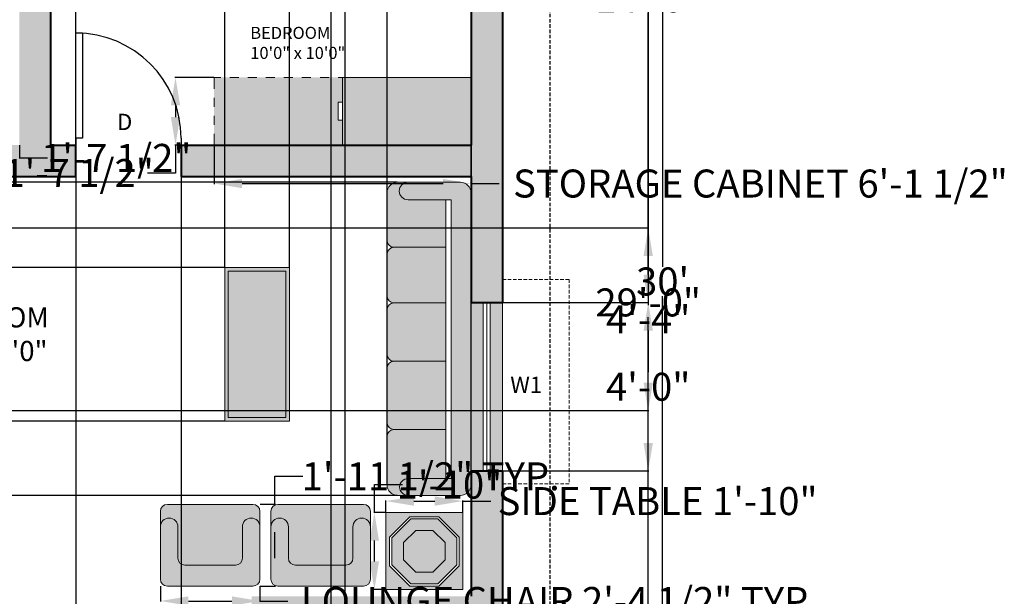
# Model space of a CAD drawing. Units: inches. Extents: x 277 to 728, y 649 to 1132.
# Tile 3 of 4: x 447 to 728, y 813 to 978. Entities that reach past the tile are written whole.
import ezdxf

# ---------------------------------------------------------------- set-up
doc = ezdxf.new("R2010")
doc.units = ezdxf.units.IN
doc.header["$MEASUREMENT"] = 0
doc.linetypes.add('DASHEDX2', pattern=[1.5, 1, -0.5])
for name, color, linetype, lineweight in [('A-ANNO-DIMS', 2, 'Continuous', 18), ('A-ANNO-TEXT', 7, 'Continuous', 18), ('A-AREA-IDEN', 7, 'Continuous', 25), ('A-DOOR', 3, 'Continuous', 25), ('A-FURN', 8, 'Continuous', 18), ('A-GLAZ', 4, 'Continuous', 18), ('A-GLAZ-OVHD', 8, 'DASHEDX2', 13), ('A-WALL', 7, 'Continuous', 40), ('A-WALL-PATT', 8, 'Continuous', 13), ('C-PROP', 7, 'DASHEDX2', 25)]:
    doc.layers.add(name, color=color, linetype=linetype, lineweight=lineweight)
doc.layers.add('A-FURN-PATT', color=9, linetype='Continuous', lineweight=9, true_color=0xd6bdce)
doc.layers.add('A-GLAZ-PATT', color=144, linetype='Continuous', lineweight=13, true_color=0x1e788f)
doc.styles.get("Standard").update_dxf_attribs({"font": 'arial.ttf'})
doc.dimstyles.get("Standard").update_dxf_attribs({"dimtxt": 8, "dimasz": 8, "dimexe": 0.18, "dimexo": 0.0625, "dimgap": 0.09, "dimtad": 0, "dimtih": 1, "dimtoh": 1, "dimdec": 0, "dimzin": 0, "dimdsep": 46, "dimlunit": 3, "dimtxsty": 'Standard', "dimcen": 0.09, "dimadec": 0, "dimazin": 0, "dimtfac": 1, "dimtdec": 0, "dimtofl": 0, "dimtmove": 0, "dimatfit": 3, "dimfxl": 1, "dimtolj": 1, "dimtzin": 0, "dimarcsym": 0})

# ---------------------------------------------------------------- blocks, each defined once
blk = doc.blocks.new('*U5')
for p, q in [((0, 0), (0, -6)), ((28, 0), (28, -6))]:
    blk.add_line(p, q)
blk.add_lwpolyline([(0, 0), (0, 28), (1.75, 28), (1.75, 0)], close=True)
blk.add_arc((0, 0), 28, 0, 90)
blk = doc.blocks.new('File Cabinet - Letter')
for p, q in [((0, 0), (15, 0)), ((0, -28.5), (0, 0)), ((15, 0), (15, -28.5)), ((15, -28.5), (0, -28.5)), ((0, -29.5), (0, -28.5)), ((5.5, -28.5), (5.5, -29.5)), ((5.5, -29.5), (9.5, -29.5)), ((9.5, -29.5), (9.5, -28.5)), ((15, -30.5), (15, -32.5)), ((0, -33.5), (0, -31.5)), ((15, -34.5), (15, -36.5)), ((0, -37.5), (0, -35.5)), ((15, -38.5), (15, -40.5)), ((0, -41.5), (0, -39.5)), ((0, -45.5), (0, -43.5)), ((15, -42.5), (15, -44.5)), ((0, -49.5), (0, -47.5)), ((15, -46.5), (15, -48.5)), ((0, -53.5), (0, -51.5)), ((15, -50.5), (15, -52.5)), ((15, -54.5), (15, -57)), ((0, -57), (0, -55.5)), ((2.5, -57), (0, -57)), ((6.5, -57), (4.5, -57)), ((10.5, -57), (8.5, -57)), ((15, -57), (12.5, -57))]:
    blk.add_line(p, q)
blk = doc.blocks.new('Hot Tub')
for p, q in [((0, 0), (0, 69.12)), ((0, 69.12), (69.12, 69.12)), ((21.601, 65.456), (3.272, 47.128)), ((22.464, 63.396), (5.358, 46.29)), ((47.521, 65.456), (21.601, 65.456)), ((46.656, 63.396), (22.464, 63.396)), ((63.763, 46.29), (46.656, 63.396)), ((65.849, 47.128), (47.521, 65.456)), ((69.12, 69.12), (69.12, 0)), ((3.272, 47.128), (3.272, 21.208)), ((5.358, 46.29), (5.358, 22.098)), ((26.785, 53.097), (15.788, 42.101)), ((42.337, 53.097), (26.785, 53.097)), ((53.333, 42.101), (42.337, 53.097)), ((63.763, 22.098), (63.763, 46.29)), ((65.849, 21.208), (65.849, 47.128)), ((15.788, 42.101), (15.788, 26.549)), ((53.333, 26.549), (53.333, 42.101)), ((3.272, 21.208), (21.601, 2.88)), ((5.358, 22.098), (22.464, 4.992)), ((15.788, 26.549), (26.785, 15.552)), ((42.337, 15.552), (53.333, 26.549)), ((46.656, 4.992), (63.763, 22.098)), ((47.521, 2.88), (65.849, 21.208)), ((26.785, 15.552), (42.337, 15.552)), ((69.12, 0), (0, 0)), ((21.601, 2.88), (47.521, 2.88)), ((22.464, 4.992), (46.656, 4.992))]:
    blk.add_line(p, q)
blk = doc.blocks.new('*D21')
at = {"layer": 'A-ANNO-DIMS', "color": 0, "lineweight": -2, "transparency": 16777216}
for p, q in [((598.28, 1083.05), (630.62, 1083.05)), ((630.44, 1075.05), (630.44, 907.23)), ((630.44, 731.05), (630.44, 898.87)), ((598.28, 723.05), (630.62, 723.05))]:
    blk.add_line(p, q, dxfattribs=at)
at = {"layer": 'A-ANNO-DIMS', "color": 0, "transparency": 16777216}
for points in [[(629.11, 1075.05), (631.77, 1075.05), (630.44, 1083.05)], [(629.11, 731.05), (631.77, 731.05), (630.44, 723.05)]]:
    blk.add_solid(points, dxfattribs=at)
at = {"layer": 'Defpoints', "color": 0, "transparency": 16777216}
for p in [(598.22, 1083.05), (598.22, 723.05), (630.44, 723.05)]:
    blk.add_point(p, dxfattribs=at)
at = {"layer": 'A-ANNO-DIMS', "color": 0, "transparency": 16777216, "insert": (630.44, 903.05), "char_height": 8, "attachment_point": 5}
blk.add_mtext("\\A1;30'", dxfattribs=at)
blk = doc.blocks.new('CHAIR-LOUNGE')
h = blk.add_hatch(color=256)
h.dxf.hatch_style = 1
h.paths.add_polyline_path([(23.44, 16.96, -1), (28.44, 16.96), (28.44, 21.37, 0.414214), (26.44, 23.37), (2, 23.37, 0.414214), (0, 21.37), (0, 16.96, -1), (5, 16.96), (5, 8, 0.414214), (7, 6), (21.44, 6, 0.414214), (23.44, 8)])
h = blk.add_hatch(color=256)
h.dxf.hatch_style = 1
h.paths.add_polyline_path([(0, 2, 0.414214), (2, 0), (26.44, 0, 0.414214), (28.44, 2), (28.44, 16.96, 1), (23.44, 16.96), (23.44, 8, -0.414214), (21.44, 6), (7, 6, -0.414214), (5, 8), (5, 16.96, 1), (0, 16.96)])
for p, q in [((2, 23.37), (26.44, 23.37)), ((0, 16.96), (0, 21.37)), ((28.44, 21.37), (28.44, 16.96)), ((0, 16.96), (0, 2)), ((5, 8), (5, 16.96)), ((23.44, 16.96), (23.44, 8)), ((28.44, 2), (28.44, 16.96)), ((21.44, 6), (7, 6)), ((2, 0), (26.44, 0))]:
    blk.add_line(p, q)
for centre, radius, start, end in [((2, 21.37), 2, 90, 180), ((26.44, 21.37), 2, 0, 90), ((2.5, 16.96), 2.5, 0, 180), ((25.94, 16.96), 2.5, 0, 180), ((7, 8), 2, 180, 270), ((21.44, 8), 2, 270, 0), ((2, 2), 2, 180, 270), ((26.44, 2), 2, 270, 0)]:
    blk.add_arc(centre, radius, start, end)
blk = doc.blocks.new('*D25')
at = {"layer": 'A-ANNO-DIMS', "color": 0, "lineweight": -2, "transparency": 16777216}
for p, q in [((551.4, 837.04), (551.4, 840.45)), ((559.4, 840.27), (565.36, 840.27)), ((573.36, 837.04), (573.36, 840.45)), ((573.36, 840.27), (581.36, 840.27))]:
    blk.add_line(p, q, dxfattribs=at)
at = {"layer": 'A-ANNO-DIMS', "color": 0, "transparency": 16777216}
for points in [[(559.4, 841.6), (559.4, 838.94), (551.4, 840.27)], [(565.36, 841.6), (565.36, 838.94), (573.36, 840.27)]]:
    blk.add_solid(points, dxfattribs=at)
at = {"layer": 'Defpoints', "color": 0, "transparency": 16777216}
for p in [(573.36, 840.27), (551.4, 836.98), (573.36, 836.98)]:
    blk.add_point(p, dxfattribs=at)
at = {"layer": 'A-ANNO-DIMS', "color": 0, "transparency": 16777216, "insert": (629.02, 840.27), "char_height": 8, "attachment_point": 5}
blk.add_mtext('\\A1;SIDE TABLE 1\'-10"', dxfattribs=at)
blk = doc.blocks.new('*D26')
at = {"layer": 'A-ANNO-DIMS', "color": 0, "lineweight": -2, "transparency": 16777216}
for p, q in [((548.11, 836.98), (548.11, 844.98)), ((548.11, 844.98), (556.11, 844.98)), ((551.34, 836.98), (547.93, 836.98)), ((548.11, 823.02), (548.11, 828.98)), ((551.34, 815.02), (547.93, 815.02))]:
    blk.add_line(p, q, dxfattribs=at)
at = {"layer": 'A-ANNO-DIMS', "color": 0, "transparency": 16777216}
for points in [[(546.77, 828.98), (549.44, 828.98), (548.11, 836.98)], [(546.77, 823.02), (549.44, 823.02), (548.11, 815.02)]]:
    blk.add_solid(points, dxfattribs=at)
at = {"layer": 'Defpoints', "color": 0, "transparency": 16777216}
for p in [(548.11, 836.98), (551.4, 836.98), (551.4, 815.02)]:
    blk.add_point(p, dxfattribs=at)
at = {"layer": 'A-ANNO-DIMS', "color": 0, "transparency": 16777216, "insert": (569.56, 844.98), "char_height": 8, "attachment_point": 5}
blk.add_mtext('\\A1;1\'-10"', dxfattribs=at)
blk = doc.blocks.new('*D29')
at = {"layer": 'A-ANNO-DIMS', "color": 0, "lineweight": -2, "transparency": 16777216}
for p, q in [((486.97, 815.91), (486.97, 811.53)), ((515.41, 815.91), (515.41, 811.53)), ((494.97, 811.71), (507.41, 811.71)), ((515.41, 811.71), (523.41, 811.71))]:
    blk.add_line(p, q, dxfattribs=at)
at = {"layer": 'A-ANNO-DIMS', "color": 0, "transparency": 16777216}
for points in [[(494.97, 813.04), (494.97, 810.37), (486.97, 811.71)], [(507.41, 813.04), (507.41, 810.37), (515.41, 811.71)]]:
    blk.add_solid(points, dxfattribs=at)
at = {"layer": 'Defpoints', "color": 0, "transparency": 16777216}
for p in [(486.97, 815.97), (515.41, 815.97), (515.41, 811.71)]:
    blk.add_point(p, dxfattribs=at)
at = {"layer": 'A-ANNO-DIMS', "color": 0, "transparency": 16777216, "insert": (601.11, 811.71), "char_height": 8, "attachment_point": 5}
blk.add_mtext('\\A1;LOUNGE CHAIR 2\'-4 1/2" TYP.', dxfattribs=at)
blk = doc.blocks.new('*D30')
at = {"layer": 'A-ANNO-DIMS', "color": 0, "lineweight": -2, "transparency": 16777216}
for p, q in [((519.67, 839.35), (519.67, 847.35)), ((519.67, 847.35), (527.67, 847.35)), ((515.47, 839.35), (519.85, 839.35)), ((519.67, 823.97), (519.67, 831.35)), ((515.47, 815.97), (519.85, 815.97))]:
    blk.add_line(p, q, dxfattribs=at)
at = {"layer": 'A-ANNO-DIMS', "color": 0, "transparency": 16777216}
for points in [[(518.34, 831.35), (521.01, 831.35), (519.67, 839.35)], [(518.34, 823.97), (521.01, 823.97), (519.67, 815.97)]]:
    blk.add_solid(points, dxfattribs=at)
at = {"layer": 'Defpoints', "color": 0, "transparency": 16777216}
for p in [(515.41, 839.35), (519.67, 839.35), (515.41, 815.97)]:
    blk.add_point(p, dxfattribs=at)
at = {"layer": 'A-ANNO-DIMS', "color": 0, "transparency": 16777216, "insert": (564.2, 847.35), "char_height": 8, "attachment_point": 5}
blk.add_mtext('\\A1;1\'-11 1/2" TYP.', dxfattribs=at)
blk = doc.blocks.new('*D32')
at = {"layer": 'A-ANNO-DIMS', "color": 0, "lineweight": -2, "transparency": 16777216}
for p, q in [((427.01, 942.02), (427, 938.24)), ((446.72, 941.99), (446.71, 938.2)), ((435, 938.4), (438.71, 938.4)), ((446.71, 938.38), (454.71, 938.37))]:
    blk.add_line(p, q, dxfattribs=at)
at = {"layer": 'A-ANNO-DIMS', "color": 0, "transparency": 16777216}
for points in [[(435, 939.74), (435, 937.07), (427, 938.42)], [(438.71, 939.73), (438.71, 937.06), (446.71, 938.38)]]:
    blk.add_solid(points, dxfattribs=at)
at = {"layer": 'Defpoints', "color": 0, "transparency": 16777216}
for p in [(427.01, 942.09), (446.72, 942.05), (446.71, 938.38)]:
    blk.add_point(p, dxfattribs=at)
at = {"layer": 'A-ANNO-DIMS', "color": 0, "transparency": 16777216, "insert": (474.38, 938.37), "char_height": 8, "attachment_point": 5}
blk.add_mtext('\\A1;1\'-7 1/2"', dxfattribs=at)
blk = doc.blocks.new('*D39')
at = {"layer": 'A-ANNO-DIMS', "color": 0, "lineweight": -2, "transparency": 16777216}
for p, q in [((502.31, 941.99), (502.31, 930.86)), ((575.72, 941.99), (575.72, 930.86)), ((510.31, 931.04), (567.72, 931.04)), ((575.72, 931.04), (583.72, 931.04))]:
    blk.add_line(p, q, dxfattribs=at)
at = {"layer": 'A-ANNO-DIMS', "color": 0, "transparency": 16777216}
for points in [[(510.31, 932.37), (510.31, 929.71), (502.31, 931.04)], [(567.72, 932.37), (567.72, 929.71), (575.72, 931.04)]]:
    blk.add_solid(points, dxfattribs=at)
at = {"layer": 'Defpoints', "color": 0, "transparency": 16777216}
for p in [(502.31, 942.05), (575.72, 942.05), (575.72, 931.04)]:
    blk.add_point(p, dxfattribs=at)
at = {"layer": 'A-ANNO-DIMS', "color": 0, "transparency": 16777216, "insert": (658.39, 931.04), "char_height": 8, "attachment_point": 5}
blk.add_mtext('\\A1;STORAGE CABINET 6\'-1 1/2"', dxfattribs=at)
blk = doc.blocks.new('*D40')
at = {"layer": 'A-ANNO-DIMS', "color": 0, "lineweight": -2, "transparency": 16777216}
for p, q in [((502.25, 961.37), (491.12, 961.37)), ((491.3, 953.37), (491.3, 950.05)), ((502.25, 942.05), (491.12, 942.05)), ((491.3, 942.05), (491.3, 934.05)), ((491.3, 934.05), (483.3, 934.05))]:
    blk.add_line(p, q, dxfattribs=at)
at = {"layer": 'A-ANNO-DIMS', "color": 0, "transparency": 16777216}
for points in [[(489.96, 953.37), (492.63, 953.37), (491.3, 961.37)], [(489.96, 950.05), (492.63, 950.05), (491.3, 942.05)]]:
    blk.add_solid(points, dxfattribs=at)
at = {"layer": 'Defpoints', "color": 0, "transparency": 16777216}
for p in [(502.31, 961.37), (491.3, 942.05), (502.31, 942.05)]:
    blk.add_point(p, dxfattribs=at)
at = {"layer": 'A-ANNO-DIMS', "color": 0, "transparency": 16777216, "insert": (463.63, 934.05), "char_height": 8, "attachment_point": 5}
blk.add_mtext('\\A1;1\'-7 1/2"', dxfattribs=at)
blk = doc.blocks.new('*D41')
at = {"layer": 'A-ANNO-DIMS', "color": 0, "lineweight": -2, "transparency": 16777216}
for p, q in [((505.29, 907.01), (299.63, 907.01)), ((299.81, 899.01), (299.81, 889.26)), ((299.81, 871.15), (299.81, 880.9)), ((505.29, 863.15), (299.63, 863.15))]:
    blk.add_line(p, q, dxfattribs=at)
at = {"layer": 'A-ANNO-DIMS', "color": 0, "transparency": 16777216}
for points in [[(298.48, 899.01), (301.15, 899.01), (299.81, 907.01)], [(298.48, 871.15), (301.15, 871.15), (299.81, 863.15)]]:
    blk.add_solid(points, dxfattribs=at)
at = {"layer": 'Defpoints', "color": 0, "transparency": 16777216}
for p in [(299.81, 907.01), (505.35, 907.01), (505.35, 863.15)]:
    blk.add_point(p, dxfattribs=at)
at = {"layer": 'A-ANNO-DIMS', "color": 0, "transparency": 16777216, "insert": (299.81, 885.08), "char_height": 8, "attachment_point": 5}
blk.add_mtext('\\A1;3\'-8"', dxfattribs=at)
blk = doc.blocks.new('*D42')
at = {"layer": 'A-ANNO-DIMS', "color": 0, "lineweight": -2, "transparency": 16777216}
for p, q in [((505.35, 907.07), (505.35, 1117.22)), ((513.35, 1117.04), (515.86, 1117.04)), ((523.86, 907.07), (523.86, 1117.22)), ((523.86, 1117.04), (531.86, 1117.04))]:
    blk.add_line(p, q, dxfattribs=at)
at = {"layer": 'A-ANNO-DIMS', "color": 0, "transparency": 16777216}
for points in [[(513.35, 1118.37), (513.35, 1115.71), (505.35, 1117.04)], [(515.86, 1118.37), (515.86, 1115.71), (523.86, 1117.04)]]:
    blk.add_solid(points, dxfattribs=at)
at = {"layer": 'Defpoints', "color": 0, "transparency": 16777216}
for p in [(523.86, 1117.04), (505.35, 907.01), (523.86, 907.01)]:
    blk.add_point(p, dxfattribs=at)
at = {"layer": 'A-ANNO-DIMS', "color": 0, "transparency": 16777216, "insert": (551.53, 1117.04), "char_height": 8, "attachment_point": 5}
blk.add_mtext('\\A1;1\'-6 1/2"', dxfattribs=at)
blk = doc.blocks.new('*D43')
at = {"layer": 'A-ANNO-DIMS', "color": 0, "lineweight": -2, "transparency": 16777216}
for p, q in [((554.66, 931.4), (299.63, 931.4)), ((299.81, 923.4), (299.81, 890.87)), ((299.81, 849.9), (299.81, 882.42)), ((554.66, 841.9), (299.63, 841.9))]:
    blk.add_line(p, q, dxfattribs=at)
at = {"layer": 'A-ANNO-DIMS', "color": 0, "transparency": 16777216}
for points in [[(298.48, 923.4), (301.15, 923.4), (299.81, 931.4)], [(298.48, 849.9), (301.15, 849.9), (299.81, 841.9)]]:
    blk.add_solid(points, dxfattribs=at)
at = {"layer": 'Defpoints', "color": 0, "transparency": 16777216}
for p in [(299.81, 931.4), (554.72, 931.4), (554.72, 841.9)]:
    blk.add_point(p, dxfattribs=at)
at = {"layer": 'A-ANNO-DIMS', "color": 0, "transparency": 16777216, "insert": (299.81, 886.65), "char_height": 8, "attachment_point": 5}
blk.add_mtext('\\A1;7\'-5 1/2"', dxfattribs=at)
blk = doc.blocks.new('*D44')
at = {"layer": 'A-ANNO-DIMS', "color": 0, "lineweight": -2, "transparency": 16777216}
for p, q in [((543.72, 1117.04), (535.72, 1117.04)), ((551.72, 844.96), (551.72, 1117.22)), ((575.72, 844.96), (575.72, 1117.22)), ((583.72, 1117.04), (591.72, 1117.04))]:
    blk.add_line(p, q, dxfattribs=at)
at = {"layer": 'A-ANNO-DIMS', "color": 0, "transparency": 16777216}
for points in [[(543.72, 1118.37), (543.72, 1115.71), (551.72, 1117.04)], [(583.72, 1118.37), (583.72, 1115.71), (575.72, 1117.04)]]:
    blk.add_solid(points, dxfattribs=at)
at = {"layer": 'Defpoints', "color": 0, "transparency": 16777216}
for p in [(575.72, 1117.04), (551.72, 844.9), (575.72, 844.9)]:
    blk.add_point(p, dxfattribs=at)
at = {"layer": 'A-ANNO-DIMS', "color": 0, "transparency": 16777216, "insert": (563.72, 1117.04), "char_height": 8, "attachment_point": 5}
blk.add_mtext('\\A1;2\'-0"', dxfattribs=at)
blk = doc.blocks.new('*D45')
at = {"layer": 'A-ANNO-DIMS', "color": 0, "lineweight": -2, "transparency": 16777216}
for p, q in [((363.23, 918.34), (626.51, 918.34)), ((626.33, 910.34), (626.33, 896.32)), ((626.33, 874.12), (626.33, 888.14)), ((363.23, 866.12), (626.51, 866.12))]:
    blk.add_line(p, q, dxfattribs=at)
at = {"layer": 'A-ANNO-DIMS', "color": 0, "transparency": 16777216}
for points in [[(625, 910.34), (627.67, 910.34), (626.33, 918.34)], [(625, 874.12), (627.67, 874.12), (626.33, 866.12)]]:
    blk.add_solid(points, dxfattribs=at)
at = {"layer": 'Defpoints', "color": 0, "transparency": 16777216}
for p in [(363.17, 918.34), (626.33, 918.34), (363.17, 866.12)]:
    blk.add_point(p, dxfattribs=at)
at = {"layer": 'A-ANNO-DIMS', "color": 0, "transparency": 16777216, "insert": (626.33, 892.23), "char_height": 8, "attachment_point": 5}
blk.add_mtext('\\A1;4\'-4"', dxfattribs=at)
blk = doc.blocks.new('*D48')
at = {"layer": 'A-ANNO-DIMS', "color": 0, "lineweight": -2, "transparency": 16777216}
for p, q in [((584.78, 1071.05), (626.51, 1071.05)), ((626.33, 1063.05), (626.33, 901.23)), ((626.33, 731.05), (626.33, 892.88)), ((584.78, 723.05), (626.51, 723.05))]:
    blk.add_line(p, q, dxfattribs=at)
at = {"layer": 'A-ANNO-DIMS', "color": 0, "transparency": 16777216}
for points in [[(625, 1063.05), (627.67, 1063.05), (626.33, 1071.05)], [(625, 731.05), (627.67, 731.05), (626.33, 723.05)]]:
    blk.add_solid(points, dxfattribs=at)
at = {"layer": 'Defpoints', "color": 0, "transparency": 16777216}
for p in [(584.72, 1071.05), (626.33, 1071.05), (584.72, 723.05)]:
    blk.add_point(p, dxfattribs=at)
at = {"layer": 'A-ANNO-DIMS', "color": 0, "transparency": 16777216, "insert": (626.33, 897.05), "char_height": 8, "attachment_point": 5}
blk.add_mtext('\\A1;29\'-0"', dxfattribs=at)
blk = doc.blocks.new('*D53')
at = {"layer": 'A-ANNO-DIMS', "color": 0, "lineweight": -2, "transparency": 16777216}
for p, q in [((584.78, 897), (626.51, 897)), ((626.33, 889), (626.33, 877.13)), ((626.33, 856.91), (626.33, 868.78)), ((584.78, 848.91), (626.51, 848.91))]:
    blk.add_line(p, q, dxfattribs=at)
at = {"layer": 'A-ANNO-DIMS', "color": 0, "transparency": 16777216}
for points in [[(625, 889), (627.67, 889), (626.33, 897)], [(625, 856.91), (627.67, 856.91), (626.33, 848.91)]]:
    blk.add_solid(points, dxfattribs=at)
at = {"layer": 'Defpoints', "color": 0, "transparency": 16777216}
for p in [(584.72, 897), (626.33, 897), (584.72, 848.91)]:
    blk.add_point(p, dxfattribs=at)
at = {"layer": 'A-ANNO-DIMS', "color": 0, "transparency": 16777216, "insert": (626.33, 872.95), "char_height": 8, "attachment_point": 5}
blk.add_mtext('\\A1;4\'-0"', dxfattribs=at)
blk = doc.blocks.new('*D54')
at = {"layer": 'A-ANNO-DIMS', "color": 0, "lineweight": -2, "transparency": 16777216}
for p, q in [((584.78, 1071.05), (626.51, 1071.05)), ((626.33, 1063.05), (626.33, 988.2)), ((626.33, 905), (626.33, 979.85)), ((584.78, 897), (626.51, 897))]:
    blk.add_line(p, q, dxfattribs=at)
at = {"layer": 'A-ANNO-DIMS', "color": 0, "transparency": 16777216}
for points in [[(625, 1063.05), (627.67, 1063.05), (626.33, 1071.05)], [(625, 905), (627.67, 905), (626.33, 897)]]:
    blk.add_solid(points, dxfattribs=at)
at = {"layer": 'Defpoints', "color": 0, "transparency": 16777216}
for p in [(584.72, 1071.05), (626.33, 1071.05), (584.72, 897)]:
    blk.add_point(p, dxfattribs=at)
at = {"layer": 'A-ANNO-DIMS', "color": 0, "transparency": 16777216, "insert": (626.33, 984.02), "char_height": 8, "attachment_point": 5}
blk.add_mtext('\\A1;14\'-6"', dxfattribs=at)
blk = doc.blocks.new('*D62')
at = {"layer": 'A-ANNO-DIMS', "color": 0, "lineweight": -2, "transparency": 16777216}
for p, q in [((462.81, 941.99), (462.81, 661.09)), ((492.89, 941.99), (492.89, 661.09)), ((454.81, 661.27), (446.81, 661.27)), ((500.89, 661.27), (508.89, 661.27))]:
    blk.add_line(p, q, dxfattribs=at)
at = {"layer": 'A-ANNO-DIMS', "color": 0, "transparency": 16777216}
for points in [[(454.81, 662.6), (454.81, 659.93), (462.81, 661.27)], [(500.89, 662.6), (500.89, 659.93), (492.89, 661.27)]]:
    blk.add_solid(points, dxfattribs=at)
at = {"layer": 'Defpoints', "color": 0, "transparency": 16777216}
for p in [(462.81, 942.05), (492.89, 942.05), (492.89, 661.27)]:
    blk.add_point(p, dxfattribs=at)
at = {"layer": 'A-ANNO-DIMS', "color": 0, "transparency": 16777216, "insert": (477.85, 661.27), "char_height": 8, "attachment_point": 5}
blk.add_mtext('\\A1;2\'-6"', dxfattribs=at)
blk = doc.blocks.new('*D64')
at = {"layer": 'A-ANNO-DIMS', "color": 0, "lineweight": -2, "transparency": 16777216}
for p, q in [((299.81, 804.05), (299.81, 812.05)), ((299.81, 812.05), (307.81, 812.05)), ((540.6, 804.05), (299.63, 804.05)), ((299.81, 792.62), (299.81, 796.05)), ((535.66, 784.62), (299.63, 784.62))]:
    blk.add_line(p, q, dxfattribs=at)
at = {"layer": 'A-ANNO-DIMS', "color": 0, "transparency": 16777216}
for points in [[(298.48, 796.05), (301.15, 796.05), (299.81, 804.05)], [(298.48, 792.62), (301.15, 792.62), (299.81, 784.62)]]:
    blk.add_solid(points, dxfattribs=at)
at = {"layer": 'Defpoints', "color": 0, "transparency": 16777216}
for p in [(299.81, 804.05), (540.67, 804.05), (535.72, 784.62)]:
    blk.add_point(p, dxfattribs=at)
at = {"layer": 'A-ANNO-DIMS', "color": 0, "transparency": 16777216, "insert": (327.48, 812.05), "char_height": 8, "attachment_point": 5}
blk.add_mtext('\\A1;1\'-7 1/2"', dxfattribs=at)
blk = doc.blocks.new('*D65')
at = {"layer": 'A-ANNO-DIMS', "color": 0, "lineweight": -2, "transparency": 16777216}
for p, q in [((447.72, 1117.04), (439.72, 1117.04)), ((455.72, 942.11), (455.72, 1117.22)), ((462.81, 942.11), (462.81, 1117.22)), ((470.81, 1117.04), (478.81, 1117.04))]:
    blk.add_line(p, q, dxfattribs=at)
at = {"layer": 'A-ANNO-DIMS', "color": 0, "transparency": 16777216}
for points in [[(447.72, 1118.37), (447.72, 1115.71), (455.72, 1117.04)], [(470.81, 1118.37), (470.81, 1115.71), (462.81, 1117.04)]]:
    blk.add_solid(points, dxfattribs=at)
at = {"layer": 'Defpoints', "color": 0, "transparency": 16777216}
for p in [(462.81, 1117.04), (455.72, 942.05), (462.81, 942.05)]:
    blk.add_point(p, dxfattribs=at)
at = {"layer": 'A-ANNO-DIMS', "color": 0, "transparency": 16777216, "insert": (489.54, 1117.04), "char_height": 8, "attachment_point": 5}
blk.add_mtext('\\A1;0\'-7"', dxfattribs=at)
blk = doc.blocks.new('*D75')
at = {"layer": 'A-ANNO-DIMS', "color": 0, "lineweight": -2, "transparency": 16777216}
for p, q in [((527.72, 1117.04), (519.72, 1117.04)), ((535.72, 784.69), (535.72, 1117.22)), ((539.72, 784.69), (539.72, 1117.22)), ((547.72, 1117.04), (555.72, 1117.04))]:
    blk.add_line(p, q, dxfattribs=at)
at = {"layer": 'A-ANNO-DIMS', "color": 0, "transparency": 16777216}
for points in [[(527.72, 1118.37), (527.72, 1115.71), (535.72, 1117.04)], [(547.72, 1118.37), (547.72, 1115.71), (539.72, 1117.04)]]:
    blk.add_solid(points, dxfattribs=at)
at = {"layer": 'Defpoints', "color": 0, "transparency": 16777216}
for p in [(535.72, 1117.04), (535.72, 784.62), (539.72, 784.62)]:
    blk.add_point(p, dxfattribs=at)
at = {"layer": 'A-ANNO-DIMS', "color": 0, "transparency": 16777216, "insert": (509, 1117.04), "char_height": 8, "attachment_point": 5}
blk.add_mtext('\\A1;0\'-4"', dxfattribs=at)

msp = doc.modelspace()

# ---------------------------------------------------------------- hatches: boundary and pattern name
at = {"layer": 'A-FURN-PATT'}
h = msp.add_hatch(color=256, dxfattribs=at)
h.dxf.hatch_style = 1
h.paths.add_polyline_path([(502.31, 942.05), (505.53, 942.05), (539.01, 942.05), (539.01, 949.13), (537.73, 949.13), (537.73, 954.29), (539.01, 954.29), (539.01, 961.37), (537.73, 961.37), (502.31, 961.37), (502.31, 958.15)])
h = msp.add_hatch(color=256, dxfattribs=at)
h.dxf.hatch_style = 1
h.paths.add_polyline_path([(575.72, 942.05), (575.72, 961.37), (539.01, 961.37), (539.01, 942.05)])
h = msp.add_hatch(color=256, dxfattribs=at)
h.dxf.hatch_style = 1
h.paths.add_polyline_path([(568.48, 912.81), (568.48, 926.4), (557.72, 926.4, -1), (557.72, 931.4), (554.72, 931.4, 0.414214), (551.72, 928.4), (551.72, 914.81, 0.414214), (553.72, 912.81)])
h = msp.add_hatch(color=256, dxfattribs=at)
h.dxf.hatch_style = 1
h.paths.add_polyline_path([(557.72, 846.7, 1), (557.72, 841.9), (572.72, 841.9, 0.414214), (575.72, 844.9), (575.72, 928.4, 0.414214), (572.72, 931.4), (557.72, 931.4, 1), (557.72, 926.4), (570, 926.4), (570, 846.7)])
h = msp.add_hatch(color=256, dxfattribs=at)
h.dxf.hatch_style = 1
h.paths.add_polyline_path([(568.48, 896.93), (568.48, 912.81), (553.72, 912.81, 0.414214), (551.72, 910.81), (551.72, 898.93, 0.414214), (553.72, 896.93)])
h = msp.add_hatch(color=256, dxfattribs=at)
h.dxf.hatch_style = 1
h.paths.add_polyline_path([(523.86, 863.15), (523.86, 907.01), (505.35, 907.01), (505.35, 863.15)])
h.paths.add_polyline_path([(506.35, 864.15), (506.35, 906.01), (522.86, 906.01), (522.86, 864.15)], flags=16)
h = msp.add_hatch(color=256, dxfattribs=at)
h.dxf.hatch_style = 1
h.paths.add_polyline_path([(506.35, 864.15), (522.86, 864.15), (522.86, 906.01), (506.35, 906.01)])
h = msp.add_hatch(color=256, dxfattribs=at)
h.dxf.hatch_style = 1
h.paths.add_polyline_path([(551.72, 882.24, 0.414214), (553.72, 880.24), (568.48, 880.24), (568.48, 896.93), (553.72, 896.93, 0.414214), (551.72, 894.93)])
h = msp.add_hatch(color=256, dxfattribs=at)
h.dxf.hatch_style = 1
h.paths.add_polyline_path([(568.48, 860.74), (568.48, 880.24), (553.72, 880.24, 0.414214), (551.72, 878.24), (551.72, 862.74, 0.414214), (553.72, 860.74)])
h = msp.add_hatch(color=256, dxfattribs=at)
h.dxf.hatch_style = 1
h.paths.add_polyline_path([(551.72, 844.9, 0.414214), (554.72, 841.9), (557.72, 841.9, -1), (557.72, 846.7), (568.48, 846.7), (568.48, 860.74), (553.72, 860.74, 0.414214), (551.72, 858.74)])
h = msp.add_hatch(color=256, dxfattribs=at)
h.dxf.hatch_style = 1
h.paths.add_polyline_path([(551.4, 815.02), (573.36, 815.02), (573.36, 836.98), (551.4, 836.98)])
h.paths.add_polyline_path([(558.26, 835.81), (566.5, 835.81), (572.32, 829.99), (572.32, 821.76), (566.5, 815.93), (558.26, 815.93), (552.44, 821.76), (552.44, 829.99)], flags=16)
h.paths.add_polyline_path([(558.54, 835.16), (566.22, 835.16), (571.66, 829.72), (571.66, 822.04), (566.22, 816.6), (558.54, 816.6), (553.1, 822.04), (553.1, 829.72)], flags=0)
h.paths.add_polyline_path([(559.91, 831.89), (564.85, 831.89), (568.34, 828.39), (568.34, 823.45), (564.85, 819.96), (559.91, 819.96), (556.41, 823.45), (556.41, 828.39)], flags=0)
h = msp.add_hatch(color=256, dxfattribs=at)
h.dxf.hatch_style = 1
h.paths.add_polyline_path([(568.34, 823.45), (568.34, 828.39), (564.85, 831.89), (559.91, 831.89), (556.41, 828.39), (556.41, 823.45), (559.91, 819.96), (564.85, 819.96)], flags=16)
h.paths.add_polyline_path([(571.66, 829.72), (566.22, 835.16), (558.54, 835.16), (553.1, 829.72), (553.1, 822.04), (558.54, 816.6), (566.22, 816.6), (571.66, 822.04)])
h = msp.add_hatch(color=256, dxfattribs=at)
h.dxf.hatch_style = 1
h.paths.add_polyline_path([(564.85, 831.89), (559.91, 831.89), (556.41, 828.39), (556.41, 823.45), (559.91, 819.96), (564.85, 819.96), (568.34, 823.45), (568.34, 828.39)])
at = {"layer": 'A-GLAZ-PATT'}
h = msp.add_hatch(color=256, dxfattribs=at)
h.dxf.hatch_style = 1
h.paths.add_polyline_path([(575.72, 848.91), (579.22, 848.91), (579.22, 897), (575.72, 897)])
h = msp.add_hatch(color=256, dxfattribs=at)
h.dxf.hatch_style = 1
h.paths.add_polyline_path([(584.72, 897), (581.22, 897), (581.22, 848.91), (584.72, 848.91)])
at = {"layer": 'A-WALL-PATT'}
h = msp.add_hatch(color=256, dxfattribs=at)
h.dxf.hatch_style = 1
h.paths.add_polyline_path([(446.72, 942.05), (422.67, 942.05), (422.67, 933.05), (462.81, 933.05), (462.81, 942.05), (455.72, 942.05), (455.72, 1062.05), (463.22, 1062.05), (463.22, 1071.05), (341.72, 1071.05), (341.72, 981.3), (350.72, 981.3), (350.72, 1062.05), (446.72, 1062.05)])
h = msp.add_hatch(color=256, dxfattribs=at)
h.dxf.hatch_style = 1
h.paths.add_polyline_path([(544.2, 933.05), (575.72, 933.05), (575.72, 897), (584.72, 897), (584.72, 1071.05), (496.36, 1071.05), (496.36, 1062.05), (575.72, 1062.05), (575.72, 942.05), (492.89, 942.05), (492.89, 933.05)])
h = msp.add_hatch(color=256, dxfattribs=at)
h.dxf.hatch_style = 1
h.paths.add_polyline_path([(513.09, 813.05), (513.09, 804.05), (575.72, 804.05), (575.72, 759.7), (584.72, 759.7), (584.72, 848.91), (575.72, 848.91), (575.72, 813.05)])

# ---------------------------------------------------------------- linework, layer by layer
at = {"layer": 'A-FURN'}
for p, q in [((572.72, 931.4), (554.72, 931.4)), ((572.72, 931.4), (557.72, 931.4)), ((551.72, 928.4), (551.72, 914.81)), ((575.72, 844.9), (575.72, 928.4)), ((557.72, 926.4), (570, 926.4)), ((568.48, 926.4), (568.48, 846.7)), ((570, 926.4), (570, 846.7)), ((553.72, 912.81), (568.48, 912.81)), ((551.72, 910.81), (551.72, 898.93)), ((551.72, 894.93), (551.72, 882.24)), ((553.72, 896.93), (568.48, 896.93)), ((551.72, 878.24), (551.72, 862.74)), ((553.72, 880.24), (568.48, 880.24)), ((553.72, 860.74), (568.48, 860.74)), ((551.72, 858.74), (551.72, 844.9)), ((570, 846.7), (557.72, 846.7)), ((554.72, 841.9), (557.72, 841.9)), ((557.72, 841.9), (572.72, 841.9))]:
    msp.add_line(p, q, dxfattribs=at)
for points in [[(505.35, 907.01), (523.86, 907.01), (523.86, 863.15), (505.35, 863.15)], [(506.35, 906.01), (522.86, 906.01), (522.86, 864.15), (506.35, 864.15)]]:
    msp.add_lwpolyline(points, close=True, dxfattribs=at)
for centre, radius, start, end in [((554.72, 928.4), 3, 90, 180), ((557.72, 928.9), 2.5, 90, 270), ((572.72, 928.4), 3, 0, 90), ((553.72, 914.81), 2, 180, 270), ((553.72, 910.81), 2, 90, 180), ((553.72, 898.93), 2, 180, 270), ((553.72, 894.93), 2, 90, 180), ((553.72, 882.24), 2, 180, 270), ((553.72, 878.24), 2, 90, 180), ((553.72, 862.74), 2, 180, 270), ((553.72, 858.74), 2, 90, 180), ((557.72, 844.3), 2.4, 90, 270), ((554.72, 844.9), 3, 180, 270), ((572.72, 844.9), 3, 270, 0)]:
    msp.add_arc(centre, radius, start, end, dxfattribs=at)
at = {"layer": 'A-GLAZ'}
for p, q in [((575.72, 897), (575.72, 848.91)), ((579.22, 897), (579.22, 848.91)), ((580.22, 897), (580.22, 848.91)), ((581.22, 897), (581.22, 848.91)), ((584.72, 897), (584.72, 848.91))]:
    msp.add_line(p, q, dxfattribs=at)
at = {"layer": 'A-GLAZ-OVHD'}
for p, q in [((584.72, 903.64), (603.73, 903.64)), ((603.73, 903.64), (603.73, 845.16)), ((603.73, 845.16), (584.72, 845.16))]:
    msp.add_line(p, q, dxfattribs=at)
at = {"layer": 'A-WALL'}
for p, q in [((584.72, 1071.05), (584.72, 897)), ((455.72, 942.05), (455.72, 1062.05)), ((575.72, 1062.05), (575.72, 942.05)), ((455.72, 942.05), (462.81, 942.05)), ((462.81, 933.05), (462.81, 942.05)), ((492.89, 942.05), (575.72, 942.05)), ((492.89, 942.05), (492.89, 933.05)), ((492.89, 942.05), (572.48, 942.05)), ((492.89, 937.55), (492.89, 933.05)), ((422.67, 933.05), (462.81, 933.05)), ((492.89, 933.05), (575.72, 933.05)), ((492.89, 933.05), (544.2, 933.05)), ((575.72, 933.05), (575.72, 897)), ((575.72, 897), (584.72, 897)), ((575.72, 848.91), (584.72, 848.91)), ((575.72, 848.91), (575.72, 813.05)), ((584.72, 848.91), (584.72, 759.7))]:
    msp.add_line(p, q, dxfattribs=at)
at = {"layer": 'C-PROP'}
msp.add_line((598.22, 1083.05), (598.22, 723.05), dxfattribs=at)

# ---------------------------------------------------------------- block references
at = {"layer": 'A-DOOR', "xscale": 1.074175063463015, "yscale": 1.074175063463015, "zscale": 1.074175063463015}
msp.add_blockref('*U5', (462.81, 944), dxfattribs=at)
at = {"layer": 'A-FURN', "xscale": 1.287891379104061, "yscale": 1.287891379104061, "zscale": 1.287891379104061, "rotation": 270}
msp.add_blockref('File Cabinet - Letter', (575.72, 961.37), dxfattribs=at)
at = {"layer": 'A-FURN'}
for p in [(486.97, 815.97), (518.55, 815.97)]:
    msp.add_blockref('CHAIR-LOUNGE', p, dxfattribs=at)
at = {"layer": 'A-FURN', "xscale": 0.3176744062489376, "yscale": 0.3176744062489376, "zscale": 0.3176744062489376}
msp.add_blockref('Hot Tub', (551.4, 815.02), dxfattribs=at)

# ---------------------------------------------------------------- texts
at = {"layer": 'A-ANNO-TEXT', "char_height": 4.66, "attachment_point": 1}
for s, insert in [('D', (474.58, 950.98)), ('W1', (586.93, 875.84))]:
    msp.add_mtext_dynamic_manual_height_columns(s, width=6.3557, gutter_width=23.3, heights=[0], dxfattribs=dict(at, insert=insert))
at = {"layer": 'A-AREA-IDEN', "attachment_point": 1}
for s, width, gutter_width, insert, char_height in [('BEDROOM\\P10\'0" x 10\'0"', 42.3466, 17.2, (512.67, 975.83), 3.4401), ('LIVING ROOM\\P  18\'9" x 10\'0"', 70.9765, 28.83, (405.77, 895.67), 5.7659)]:
    msp.add_mtext_dynamic_manual_height_columns(s, width=width, gutter_width=gutter_width, heights=[0], dxfattribs=dict(at, insert=insert, char_height=char_height))

# ---------------------------------------------------------------- dimensions: what is measured, and where the dimension line sits
at = {"layer": 'A-ANNO-DIMS'}
for base, p1, p2, picture, middle in [((523.86, 1117.04), (505.35, 907.01), (523.86, 907.01), '*D42', (551.53, 1117.04)), ((462.81, 1117.04), (455.72, 942.05), (462.81, 942.05), '*D65', (489.54, 1117.04)), ((535.72, 1117.04), (539.72, 784.62), (535.72, 784.62), '*D75', (509, 1117.04)), ((575.72, 1117.04), (551.72, 844.9), (575.72, 844.9), '*D44', (563.72, 1117.04)), ((492.89, 661.27), (462.81, 942.05), (492.89, 942.05), '*D62', (477.85, 661.27))]:
    dim = msp.add_linear_dim(base=base, p1=p1, p2=p2, dimstyle='Standard', override={"dimdec": 1, "dimlfac": 1, "dimrnd": 0, "dimzin": 1, "dimdsep": 46, "dimlunit": 4, "dimfrac": 2}, dxfattribs=at)
    dim.commit()
    dim.dimension.update_dxf_attribs({"geometry": picture, "text_midpoint": middle})
for base, p1, p2, angle, override, picture, middle in [((630.44, 723.05), (598.22, 1083.05), (598.22, 723.05), 90, {"dimclrd": 0, "dimclre": 0, "dimclrt": 0}, '*D21', (630.44, 903.05)), ((626.33, 1071.05), (584.72, 723.05), (584.72, 1071.05), 90, {"dimdec": 1, "dimlfac": 1, "dimrnd": 0, "dimzin": 1, "dimdsep": 46, "dimlunit": 4, "dimfrac": 2}, '*D48', (626.33, 897.05)), ((626.3327, 1071.0508), (584.7185, 896.9974), (584.7185, 1071.0508), 90, {"dimdec": 1, "dimlfac": 1, "dimrnd": 0, "dimzin": 1, "dimdsep": 46, "dimlunit": 4, "dimfrac": 2}, '*D54', (626.3327, 984.0241)), ((491.3, 942.05), (502.31, 961.37), (502.31, 942.05), 270, {"dimdec": 1, "dimlfac": 1, "dimrnd": 0, "dimzin": 1, "dimdsep": 46, "dimlunit": 4, "dimfrac": 2}, '*D40', (463.63, 934.05)), ((446.71, 938.38), (427.01, 942.09), (446.72, 942.05), 359.8953, {"dimdec": 1, "dimlfac": 1, "dimrnd": 0, "dimzin": 1, "dimdsep": 46, "dimlunit": 4, "dimfrac": 2}, '*D32', (474.38, 938.37)), ((299.81, 931.4), (554.72, 841.9), (554.72, 931.4), 90, {"dimdec": 1, "dimlfac": 1, "dimrnd": 0, "dimzin": 1, "dimdsep": 46, "dimlunit": 4, "dimfrac": 2}, '*D43', (299.81, 886.65)), ((626.33, 918.34), (363.17, 866.12), (363.17, 918.34), 90, {"dimdec": 1, "dimlfac": 1, "dimrnd": 0, "dimzin": 1, "dimdsep": 46, "dimlunit": 4, "dimfrac": 2}, '*D45', (626.33, 892.23)), ((299.81, 907.01), (505.35, 863.15), (505.35, 907.01), 90, {"dimdec": 1, "dimlfac": 1, "dimrnd": 0, "dimzin": 1, "dimdsep": 46, "dimlunit": 4, "dimfrac": 2}, '*D41', (299.81, 885.08)), ((626.33, 897), (584.72, 848.91), (584.72, 897), 90, {"dimdec": 1, "dimlfac": 1, "dimrnd": 0, "dimzin": 1, "dimdsep": 46, "dimlunit": 4, "dimfrac": 2}, '*D53', (626.33, 872.95)), ((548.11, 836.98), (551.4, 815.02), (551.4, 836.98), 90, {"dimdec": 1, "dimlfac": 1, "dimrnd": 0, "dimzin": 1, "dimdsep": 46, "dimlunit": 4, "dimfrac": 2}, '*D26', (569.56, 844.98)), ((299.81, 804.05), (535.72, 784.62), (540.67, 804.05), 90, {"dimdec": 1, "dimlfac": 1, "dimrnd": 0, "dimzin": 1, "dimdsep": 46, "dimlunit": 4, "dimfrac": 2}, '*D64', (327.48, 812.05))]:
    dim = msp.add_linear_dim(base=base, p1=p1, p2=p2, angle=angle, dimstyle='Standard', override=override, dxfattribs=at)
    dim.commit()
    dim.dimension.update_dxf_attribs({"geometry": picture, "text_midpoint": middle})
for base, p1, p2, text, picture, middle in [((575.72, 931.04), (502.31, 942.05), (575.72, 942.05), 'STORAGE CABINET <>', '*D39', (658.39, 931.04)), ((573.36, 840.27), (551.4, 836.98), (573.36, 836.98), 'SIDE TABLE <>', '*D25', (629.02, 840.27)), ((515.41, 811.71), (486.97, 815.97), (515.41, 815.97), 'LOUNGE CHAIR <> TYP.', '*D29', (601.11, 811.71))]:
    dim = msp.add_linear_dim(base=base, p1=p1, p2=p2, text=text, dimstyle='Standard', override={"dimdec": 1, "dimlfac": 1, "dimrnd": 0, "dimzin": 1, "dimdsep": 46, "dimlunit": 4, "dimfrac": 2}, dxfattribs=at)
    dim.commit()
    dim.dimension.update_dxf_attribs({"geometry": picture, "text_midpoint": middle})
dim = msp.add_linear_dim(base=(519.67, 839.35), p1=(515.41, 815.97), p2=(515.41, 839.35), angle=90, text='<> TYP.', dimstyle='Standard', override={"dimdec": 1, "dimlfac": 1, "dimrnd": 0, "dimzin": 1, "dimdsep": 46, "dimlunit": 4, "dimfrac": 2}, dxfattribs=at)
dim.commit()
dim.dimension.update_dxf_attribs({"geometry": '*D30', "text_midpoint": (564.2, 847.35)})

doc.saveas('drawing.dxf')
